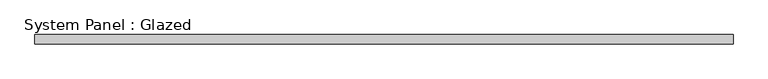
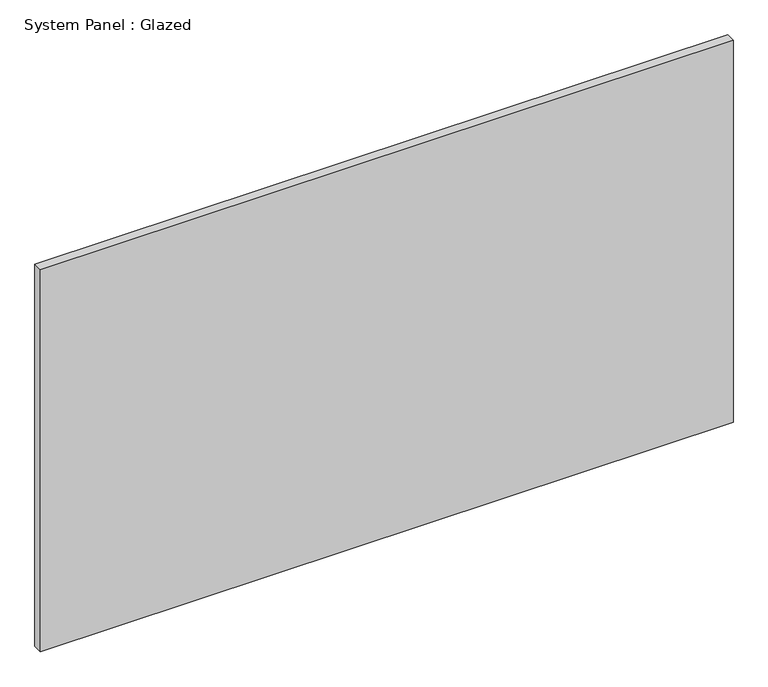
"""IFC4 building model written with IfcOpenShell, lengths in millimetres: plate geometry, System Panel : Glazed."""

from ifc_helpers import new_model, si_unit, origin, origin_with_axes, place, context, project, spatial, polyline, outline, extrude, source, transform, mapped, element, save


def system_panel_glazed_442d96c1(model_context):
    return source(origin(), model_context, "Body", "SweptSolid", [
        extrude(outline(polyline([(915.0000002, 24.5), (-915.0000002, 24.5), (-915.0000002, 49.5), (915.0000002, 49.5), (915.0000002, 24.5)])), origin_with_axes(), (0.0, 0.0, 1.0), 1067.1518548),
    ])


if __name__ == "__main__":
    model = new_model("IFC4")
    model_context = context("Model", 3, world=origin())
    ifc_project = project(units=[si_unit("LENGTHUNIT", "METRE", prefix="MILLI")], contexts=[model_context])
    site = spatial("IfcSite", under=ifc_project)
    building = spatial("IfcBuilding", under=site)
    placement = place(None, origin())
    system_panel_glazed_shape = system_panel_glazed_442d96c1(model_context)
    element("IfcPlate", 1, ObjectType="System Panel : Glazed", at=placement, inside=building, context=model_context, shape_type="MappedRepresentation", body=[
        mapped(system_panel_glazed_shape, transform((0.0, 0.0, 0.0), x_axis=(1.0, 0.0, 0.0), y_axis=(0.0, 1.0, 0.0), z_axis=(0.0, 0.0, 1.0))),
    ])
    save(model, "model.ifc")

# Revit data of these elements
# Type "System Panel : Glazed"
#   Keynote = "H11"
#   Construction Type Id = "GSP4R"
#   Analytic Construction = "1/8 in Pilkington single glazing"
#   Visual Light Transmittance = 0.9
#   Solar Heat Gain Coefficient = 0.86
#   Heat Transfer Coefficient (U) = 6.7069 W/(m²·K)
#   Define Thermal Properties by = 1
# Element 1 (IfcPlate, "System Panel : Glazed")
#   Materials on its faces: "Glass"
# Materials
#   "Glass": class "Glass", colour RGB 0 128 192, transparency 0.9, Description = "Soda Lime Glass", Cost = 0
